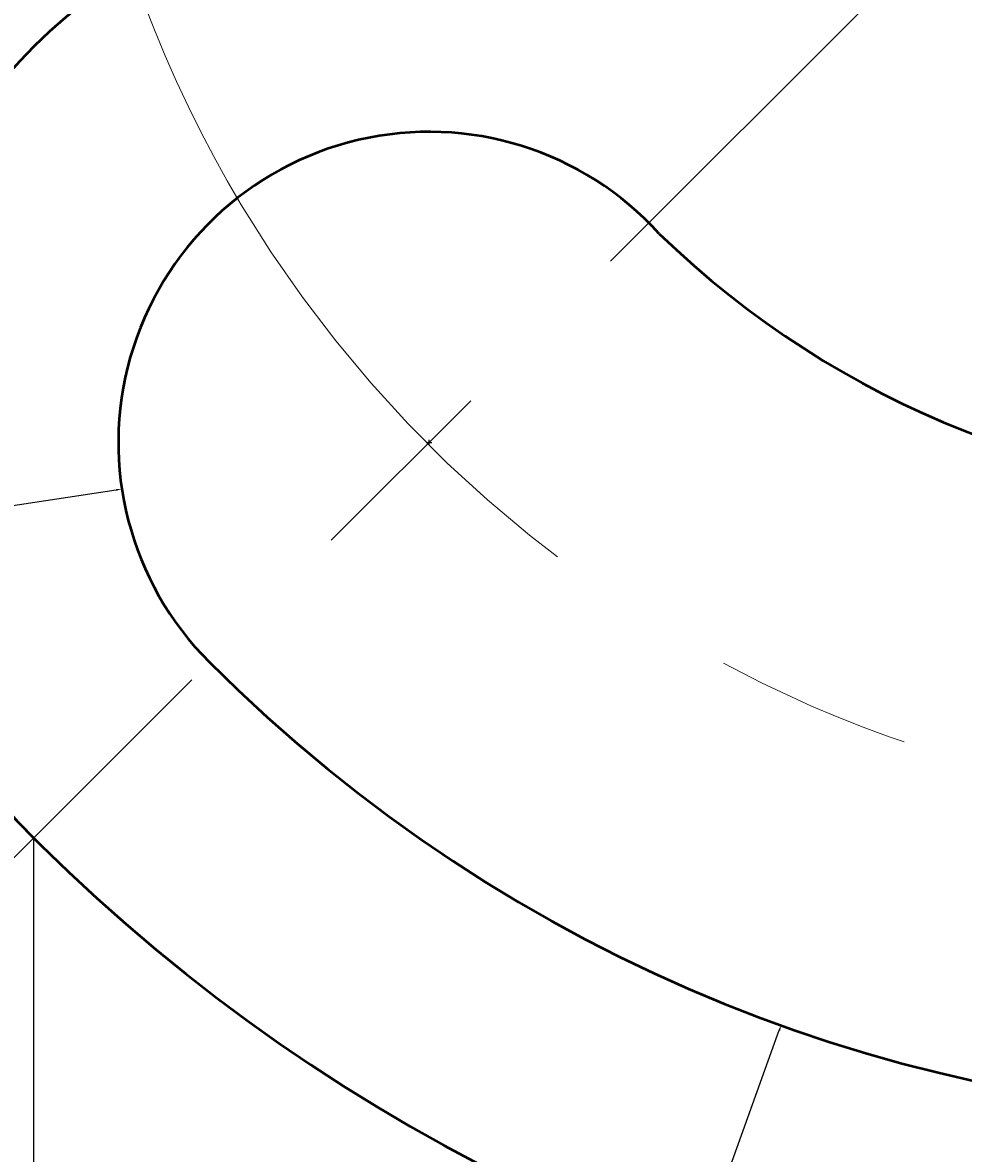
# Model space of a CAD drawing. Units: millimetres. Extents: x -53 to 92, y -147 to 37.
# Tile 3 of 16: x -22 to 8, y -105 to -69. Entities that reach past the tile are written whole.
import ezdxf

# ---------------------------------------------------------------- set-up
doc = ezdxf.new("R2010")
doc.units = ezdxf.units.MM
doc.header["$MEASUREMENT"] = 0
doc.linetypes.add('CENTER', pattern=[50.8, 31.75, -6.35, 6.35, -6.35])
for name, color, linetype, lineweight in [('M-CNTR', 4, 'CENTER', 18), ('M-DIMS', 2, 'Continuous', 25), ('M-OUTL', 7, 'Continuous', 50)]:
    doc.layers.add(name, color=color, linetype=linetype, lineweight=lineweight)
doc.styles.get("Standard").update_dxf_attribs({"font": 'arial.ttf'})
doc.dimstyles.get("Standard").update_dxf_attribs({"dimtxt": 0.18, "dimasz": 0.18, "dimexe": 0.18, "dimexo": 0.0625, "dimgap": 0.09, "dimtad": 0, "dimtih": 1, "dimtoh": 1, "dimdec": 4, "dimzin": 0, "dimdsep": 46, "dimtxsty": 'Standard', "dimcen": 0.09, "dimadec": 0, "dimazin": 0, "dimtfac": 1, "dimtdec": 4, "dimtofl": 0, "dimtmove": 0, "dimatfit": 3, "dimfxl": 1, "dimtolj": 1, "dimtzin": 0, "dimarcsym": 0})

# ---------------------------------------------------------------- blocks, each defined once
blk = doc.blocks.new('*D8')
at = {"layer": 'Defpoints', "color": 0, "transparency": 16777216}
for p in [(-9.328, -82.264), (-19.215, -83.763)]:
    blk.add_point(p, dxfattribs=at)
at = {"layer": 'M-DIMS', "color": 0, "lineweight": -2, "transparency": 16777216}
for p, q in [((-9.328, -82.354), (-9.328, -82.174)), ((-9.418, -82.264), (-9.238, -82.264)), ((-46.381, -87.879), (-19.393, -83.79))]:
    blk.add_line(p, q, dxfattribs=at)
at = {"layer": 'M-DIMS', "color": 0, "transparency": 16777216}
blk.add_solid([(-19.397, -83.76), (-19.388, -83.819), (-19.215, -83.763)], dxfattribs=at)
at = {"layer": 'M-DIMS', "color": 0, "transparency": 16777216, "insert": (-50.05, -87.879), "char_height": 0.18, "attachment_point": 5}
blk.add_mtext('\\A1;{\\H16.66667x;R10}', dxfattribs=at)
blk = doc.blocks.new('*D10')
at = {"layer": 'Defpoints', "color": 0, "transparency": 16777216}
for p in [(64.593, -18.184), (-26.68, -89.776)]:
    blk.add_point(p, dxfattribs=at)
at = {"layer": 'M-DIMS', "color": 0, "lineweight": -2, "transparency": 16777216}
for p, q in [((77.384, -8.151), (64.734, -18.073)), ((77.564, -8.151), (77.384, -8.151)), ((18.866, -53.98), (19.046, -53.98)), ((18.956, -54.07), (18.956, -53.89))]:
    blk.add_line(p, q, dxfattribs=at)
at = {"layer": 'M-DIMS', "color": 0, "transparency": 16777216}
blk.add_solid([(64.716, -18.05), (64.753, -18.097), (64.593, -18.184)], dxfattribs=at)
at = {"layer": 'M-DIMS', "color": 0, "transparency": 16777216, "insert": (82.599, -8.151), "char_height": 0.18, "attachment_point": 5}
blk.add_mtext('\\A1;{\\H16.66667x;%%C116}', dxfattribs=at)
blk = doc.blocks.new('*D16')
at = {"layer": 'Defpoints', "color": 0, "transparency": 16777216}
for p in [(-22.056, -94.992), (59.969, -94.992), (59.969, -138.812)]:
    blk.add_point(p, dxfattribs=at)
at = {"layer": 'M-DIMS', "color": 0, "lineweight": -2, "transparency": 16777216}
for p, q in [((-22.056, -95.055), (-22.056, -138.992)), ((59.969, -95.055), (59.969, -138.992)), ((-21.876, -138.812), (18.563, -138.812)), ((59.789, -138.812), (19.349, -138.812))]:
    blk.add_line(p, q, dxfattribs=at)
at = {"layer": 'M-DIMS', "color": 0, "transparency": 16777216}
for points in [[(-21.876, -138.782), (-21.876, -138.842), (-22.056, -138.812)], [(59.789, -138.782), (59.789, -138.842), (59.969, -138.812)]]:
    blk.add_solid(points, dxfattribs=at)
at = {"layer": 'M-DIMS', "color": 0, "transparency": 16777216, "insert": (18.956, -138.812), "char_height": 0.18, "attachment_point": 5}
blk.add_mtext('\\A1;82.02', dxfattribs=at)
blk = doc.blocks.new('*D17')
at = {"layer": 'Defpoints', "color": 0, "transparency": 16777216}
for p in [(-46.81, 25.909), (28.564, 25.909), (18.165, -111.975)]:
    blk.add_point(p, dxfattribs=at)
at = {"layer": 'M-DIMS', "color": 0, "lineweight": -2, "transparency": 16777216}
for p, q in [((28.502, 25.909), (-46.99, 25.909)), ((-46.81, 25.729), (-46.81, -42.851)), ((-46.81, -111.795), (-46.81, -43.215)), ((18.102, -111.975), (-46.99, -111.975))]:
    blk.add_line(p, q, dxfattribs=at)
at = {"layer": 'M-DIMS', "color": 0, "transparency": 16777216}
for points in [[(-46.84, 25.729), (-46.78, 25.729), (-46.81, 25.909)], [(-46.84, -111.795), (-46.78, -111.795), (-46.81, -111.975)]]:
    blk.add_solid(points, dxfattribs=at)
at = {"layer": 'M-DIMS', "color": 0, "transparency": 16777216, "insert": (-46.81, -43.033), "char_height": 0.18, "attachment_point": 5}
blk.add_mtext('\\A1;137.88', dxfattribs=at)
blk = doc.blocks.new('*D22')
at = {"layer": 'Defpoints', "color": 0, "transparency": 16777216}
for p in [(-27.328, -82.26), (-9.328, -82.264)]:
    blk.add_point(p, dxfattribs=at)
at = {"layer": 'M-DIMS', "color": 0, "lineweight": -2, "transparency": 16777216}
for p, q in [((-9.328, -82.354), (-9.328, -82.174)), ((-38.128, -82.257), (-27.508, -82.26)), ((-9.418, -82.264), (-9.238, -82.264))]:
    blk.add_line(p, q, dxfattribs=at)
at = {"layer": 'M-DIMS', "color": 0, "transparency": 16777216}
blk.add_solid([(-27.508, -82.23), (-27.508, -82.29), (-27.328, -82.26)], dxfattribs=at)
at = {"layer": 'M-DIMS', "color": 0, "transparency": 16777216, "insert": (-38.628, -82.257), "char_height": 0.18, "attachment_point": 5}
blk.add_mtext('\\A1;2X R18', dxfattribs=at)
blk = doc.blocks.new('*D24')
at = {"layer": 'Defpoints', "color": 0, "transparency": 16777216}
for p in [(18.956, -53.969), (2.002, -101.015)]:
    blk.add_point(p, dxfattribs=at)
at = {"layer": 'M-DIMS', "color": 0, "lineweight": -2, "transparency": 16777216}
for p, q in [((18.866, -53.969), (19.046, -53.969)), ((18.956, -54.059), (18.956, -53.879)), ((-8.171, -129.243), (1.941, -101.184)), ((-8.351, -129.243), (-8.171, -129.243))]:
    blk.add_line(p, q, dxfattribs=at)
at = {"layer": 'M-DIMS', "color": 0, "transparency": 16777216}
blk.add_solid([(1.912, -101.174), (1.969, -101.195), (2.002, -101.015)], dxfattribs=at)
at = {"layer": 'M-DIMS', "color": 0, "transparency": 16777216, "insert": (-8.813, -129.243), "char_height": 0.18, "attachment_point": 5}
blk.add_mtext('\\A1;R50.01', dxfattribs=at)

msp = doc.modelspace()

# ---------------------------------------------------------------- linework, layer by layer
at = {"layer": 'M-CNTR'}
msp.add_line((18.95638, -53.98007), (-27.00556, -99.94201), dxfattribs=at)
msp.add_arc((18.95638, -54.07007), 40, 187.365915, 352.627832, dxfattribs=at)
at = {"layer": 'M-OUTL'}
for centre, radius, start, end in [((18.95638, -53.98007), 58, 108.3895553, 70.0459142), ((-9.32787, -82.26433), 18, 84.624123, 224.999991), ((-9.32787, -82.26433), 10, 42.208735, 224.999984), ((18.95638, -53.98007), 30.01579, 224.070398, 224.071058), ((18.95638, -53.98007), 30.01579, 225.928942, 314.071058), ((18.95621, -53.96903), 50.00792, 225.009078, 314.99431)]:
    msp.add_arc(centre, radius, start, end, dxfattribs=at)

# ---------------------------------------------------------------- dimensions: what is measured, and where the dimension line sits
at = {"layer": 'M-DIMS'}
dim = msp.add_linear_dim(base=(-46.8103, 25.90924), p1=(18.16452, -111.97467), p2=(28.56407, 25.90924), angle=90, dimstyle='Standard', override={"dimdec": 2, "dimlfac": 1, "dimrnd": 0, "dimzin": 0, "dimdsep": 46, "dimlunit": 2}, dxfattribs=at)
dim.commit()
dim.dimension.update_dxf_attribs({"geometry": '*D17', "text_midpoint": (-46.8103, -43.03271)})
dim = msp.add_diameter_dim_2p(p1=(-26.67986, -89.77579), p2=(64.59262, -18.18435), text='{\\H16.66667x;%%C116}', dimstyle='Standard', override={"dimclrd": 0, "dimclre": 0, "dimclrt": 0}, dxfattribs=at)
dim.commit()
dim.dimension.update_dxf_attribs({"geometry": '*D10', "text_midpoint": (82.59889, -8.15132), "dimtype": 163})
dim = msp.add_radius_dim(center=(18.95621, -53.96903), mpoint=(2.00175, -101.01516), dimstyle='Standard', override={"dimdec": 2, "dimlfac": 1, "dimrnd": 0, "dimzin": 0, "dimdsep": 46, "dimlunit": 2}, dxfattribs=at)
dim.commit()
dim.dimension.update_dxf_attribs({"geometry": '*D24', "text_midpoint": (-8.8134, -129.24283), "dimtype": 164})
for mpoint, text, override, picture, middle in [((-19.215, -83.76259), '{\\H16.66667x;R10}', {"dimclrd": 0, "dimclre": 0, "dimclrt": 0}, '*D8', (-46.38072, -87.8792)), ((-27.32787, -82.26), '2X <>', {"dimdec": 0, "dimlfac": 1, "dimrnd": 0, "dimzin": 0, "dimdsep": 46, "dimlunit": 2}, '*D22', (-38.12787, -82.2574))]:
    dim = msp.add_radius_dim(center=(-9.32787, -82.26433), mpoint=mpoint, text=text, dimstyle='Standard', override=override, dxfattribs=at)
    dim.commit()
    dim.dimension.update_dxf_attribs({"geometry": picture, "text_midpoint": middle, "dimtype": 164})
dim = msp.add_linear_dim(base=(59.96857, -138.81235), p1=(-22.0558, -94.99225), p2=(59.96857, -94.99226), dimstyle='Standard', override={"dimdec": 2, "dimlfac": 1, "dimrnd": 0, "dimzin": 0, "dimdsep": 46, "dimlunit": 2}, dxfattribs=at)
dim.commit()
dim.dimension.update_dxf_attribs({"geometry": '*D16', "text_midpoint": (18.95639, -138.81235)})

doc.saveas('drawing.dxf')
